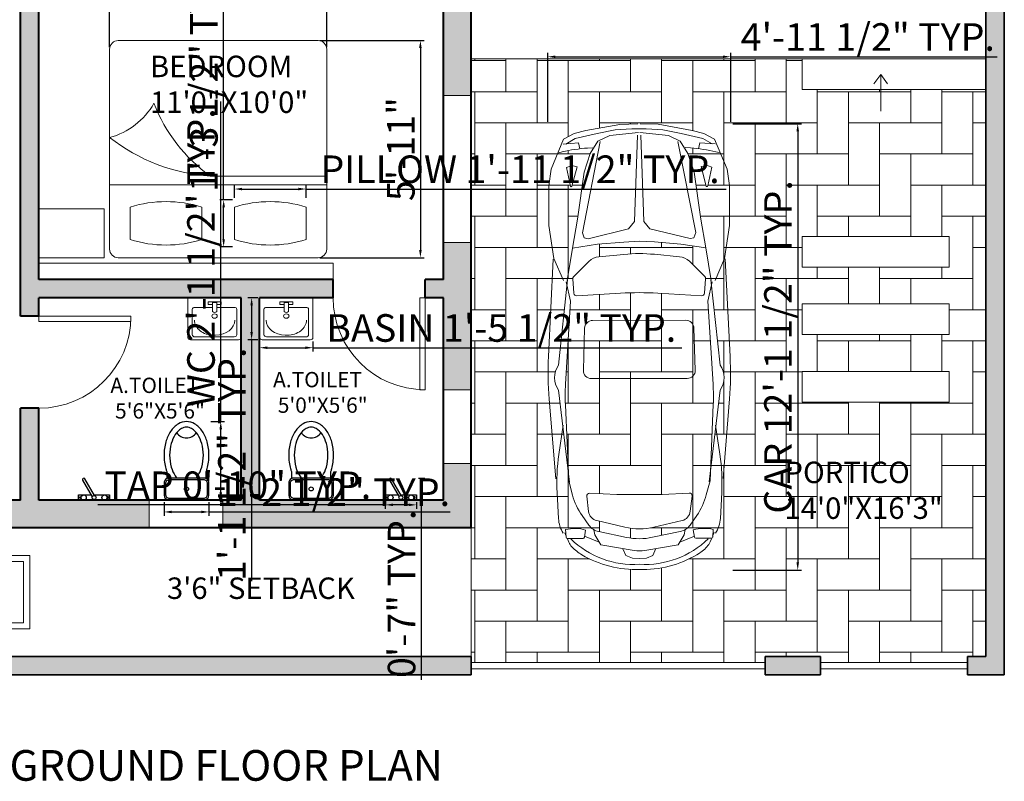
# Model space of a CAD drawing. Units: inches. Extents: x 2337 to 3570, y 1258 to 1938.
# Tile 2 of 30: x 2585 to 2906, y 1258 to 1507. Entities that reach past the tile are written whole.
import ezdxf

# ---------------------------------------------------------------- set-up
doc = ezdxf.new("R2010")
doc.units = ezdxf.units.IN
for name, color, linetype, lineweight in [('A-ANNO-DIMS', 2, 'Continuous', 18), ('A-ANNO-SYMB', 7, 'Continuous', 18), ('A-ANNO-TEXT', 7, 'Continuous', 18), ('A-ANNO-TITL', 7, 'Continuous', 30), ('A-AREA-IDEN', 7, 'Continuous', 18), ('A-DOOR', 4, 'Continuous', 20), ('A-FLOR-EDGE', 8, 'Continuous', 20), ('A-FLOR-PATT', 252, 'Continuous', 13), ('A-FLOR-STRS', 7, 'Continuous', 20), ('A-GLAZ', 4, 'Continuous', 18), ('A-WALL', 7, 'Continuous', 40), ('C-PROP', 7, 'Continuous', 35), ('furn', 8, 'Continuous', 18), ('L-PLNT-BEDS', 94, 'Continuous', 20), ('L-SITE-GATE', 4, 'Continuous', 18), ('L-SITE-VEHI', 8, 'Continuous', 18), ('Сантехника', 9, 'Continuous', 18)]:
    doc.layers.add(name, color=color, linetype=linetype, lineweight=lineweight)
doc.layers.add('A-WALL-PATT', color=18, linetype='Continuous', lineweight=13, true_color=0x000000)
doc.layers.add('C-PROP-PATT', color=251, linetype='Continuous', lineweight=13, true_color=0x636466)
doc.layers.add('SANTEH', color=7, linetype='Continuous')
doc.styles.get("Standard").update_dxf_attribs({"font": 'arial.ttf'})
doc.dimstyles.new('ISO-25', dxfattribs={"dimtxt": 9, "dimasz": 2.5, "dimexe": 1.25, "dimexo": 0.625, "dimtad": 1, "dimdec": 1, "dimlunit": 3, "dimtxsty": 'Standard', "dimcen": 2.5, "dimadec": 0, "dimazin": 0, "dimtfac": 1, "dimtdec": 1, "dimtmove": 0, "dimatfit": 3, "dimfxl": 1, "dimarcsym": 0})

# ---------------------------------------------------------------- blocks, each defined once
blk = doc.blocks.new('*U3')
for p, q in [((0, 0), (0, -6)), ((30, 0), (30, -6))]:
    blk.add_line(p, q)
blk.add_lwpolyline([(0, 0), (0, 30), (1.75, 30), (1.75, 0)], close=True)
blk.add_arc((0, 0), 30, 0, 90)
blk = doc.blocks.new('Rac7')
at = {"color": 0}
for p, q in [((-39473.6, -23808.4), (-38988.3, -23808.4)), ((-39500.6, -24232.1), (-39500.6, -23829.6)), ((-39456.5, -23859.1), (-39456.5, -24114.9)), ((-39032.4, -23838), (-39429.6, -23838)), ((-39221.1, -23854.9), (-39240.8, -23854.9)), ((-39005.4, -24114.9), (-39005.4, -23859.1)), ((-39005.4, -23859.1), (-39005.4, -23859.1)), ((-38961.3, -23829.6), (-38961.3, -24232.1)), ((-39252.5, -24185.9), (-39252.5, -24093.6)), ((-39209.4, -24185.9), (-39209.4, -24093.6)), ((-39429.6, -24136.1), (-39252.5, -24136.1)), ((-39297, -24164), (-39252.5, -24164)), ((-39297, -24193.5), (-39297, -24164)), ((-39164.9, -24193.5), (-39297, -24193.5)), ((-39252.5, -24185.9), (-39209.4, -24185.9)), ((-39209.4, -24136.1), (-39032.4, -24136.1)), ((-39209.4, -24164), (-39164.9, -24164)), ((-39164.9, -24164), (-39164.9, -24193.5)), ((-38961.3, -24232.1), (-39500.6, -24232.1))]:
    blk.add_line(p, q, dxfattribs=at)
at = {"color": 0, "extrusion": (0, 0, -1)}
for centre, major_axis, start_param, end_param in [((-39473.6, -23829.6), (-27, 0), 0, 1.570796), ((-38988.3, -23829.6), (-27, 0), 1.570796, 3.141593), ((-39429.6, -23859.1), (-27, 0), 0, 1.570796), ((-39240.8, -24007.4), (-194.1, 0), 0, 1.570796), ((-39221.1, -24007.4), (-194.1, 0), 1.570796, 3.141593), ((-39032.4, -23859.1), (-27, 0), 1.570796, 3.141593), ((-39231, -24104), (-25.3, 0), 0.552816, 2.588777), ((-39429.6, -24114.9), (-27, 0), -1.570796, 0), ((-39032.4, -24114.9), (-27, 0), -3.141593, -1.570796)]:
    blk.add_ellipse(centre, major_axis=major_axis, ratio=0.785714, start_param=start_param, end_param=end_param, dxfattribs=at)
blk.add_ellipse((-39231, -24048), major_axis=(-27.9, 0), ratio=0.785714, dxfattribs=at)
blk = doc.blocks.new('K10-44')
at = {"layer": 'SANTEH'}
for points in [[(-182, 222.6, 0.020439), (-174, 197.6), (-174, 134.8, 0.262987), (-198.2, 92), (-198.2, -8, 0.414214), (-148.2, -58), (151.8, -58, 0.414214), (201.8, -8), (201.8, 92, 0.262987), (177.6, 134.8), (177.6, 197.6, 0.020439), (185.6, 222.6, 0.067459), (201.8, 342, 0.067459), (185.6, 461.3, 0.079812), (143.2, 554.1, 0.107118), (73.7, 621.5, 0.139889), (1.8, 642, 0.139889), (-70.1, 621.5, 0.107118), (-139.6, 554.1, 0.079812), (-182, 461.3, 0.067459), (-198.2, 342, 0.067459)], [(-148.2, 127), (151.8, 127, -0.414214), (186.8, 92), (186.8, -8, -0.414214), (151.8, -43), (-148.2, -43, -0.414214), (-183.2, -8), (-183.2, 92, -0.414214)]]:
    blk.add_lwpolyline(points, format="xyb", close=True, dxfattribs=at)
for points in [[(89.9, 142, 0.027307), (101.6, 157.6, 0.079812), (137.4, 235.9, 0.067459), (151.8, 342, 0.067459), (137.4, 448, 0.079812), (101.6, 526.4, 0.107118), (47.3, 579, 0.139889), (1.8, 592, 0.139889), (-43.7, 579, 0.107118), (-98, 526.4, 0.079812), (-133.8, 448, 0.067459), (-148.2, 342, 0.067459), (-133.8, 235.9, 0.079812), (-98, 157.6, 0.027307), (-86.4, 142, 0.139889)], [(-174, 134.8, -0.136371), (-148.2, 142), (151.8, 142, -0.136371), (177.6, 134.8)]]:
    blk.add_lwpolyline(points, format="xyb", dxfattribs=at)
blk.add_circle((1.8, 42), 18.3, dxfattribs=at)
blk.add_arc((1.8, 601.6), 105.3, 213.89944, 326.10056, dxfattribs=at)
blk = doc.blocks.new('Faucet - kit sink top')
at = {"layer": 'SANTEH'}
for p, q in [((-5.5, -0.75), (-5.5, -1.25)), ((-4.94278, -0.75), (-5.5, -0.75)), ((-5.5, -1.25), (-4.94278, -1.25)), ((-0.14775, -1.7441), (3.56698, -8.1782)), ((4.43301, -7.6782), (0.71828, -1.2441)), ((4.94278, -0.75), (5.5, -0.75)), ((5.5, -1.25), (4.94278, -1.25)), ((5.5, -0.75), (5.5, -1.25))]:
    blk.add_line(p, q, dxfattribs=at)
blk.add_lwpolyline([(-0.00587, -2), (-6, -2), (-6, 0), (6, 0), (6, -2), (1.15195, -2)], dxfattribs=at)
for centre, radius in [((-4, -1), 1), ((4, -1), 1), ((0, -1), 0.75)]:
    blk.add_circle(centre, radius, dxfattribs=at)
blk.add_arc((4, -7.9282), 0.5, 210, 30, dxfattribs=at)
blk = doc.blocks.new('A$C4A3239E3')
for p, q in [((1.2507, 1.6335), (2.1522, 1.6799)), ((2.5445, 1.6742), (3.2816, 1.6148)), ((0.2661, 1.5794), (0.2592, 1.5495)), ((1.4425, 1.5023), (2.2313, 1.5881)), ((2.4629, 1.587), (3.3117, 1.4863)), ((2.7875, 1.5463), (3.0567, 1.5859)), ((3.4104, 1.6024), (3.6491, 1.5899)), ((0.1359, 1.4288), (0.1867, 1.515)), ((0.1752, 1.399), (0.1867, 1.5408)), ((0.3898, 1.477), (0.4021, 1.5106)), ((0.5758, 1.4596), (0.3963, 1.4117)), ((0.4021, 1.5106), (0.5754, 1.4741)), ((1.4497, 1.5063), (1.149, 1.4553)), ((1.4612, 1.5146), (1.6407, 1.4739)), ((1.6407, 1.4739), (2.4076, 1.5225)), ((2.597, 1.5244), (3.3012, 1.4943)), ((3.3012, 1.4943), (3.4322, 1.4598)), ((3.8218, 1.5205), (3.7519, 1.525)), ((3.7813, 1.5317), (3.8128, 1.5185)), ((3.8334, 1.3629), (3.8334, 1.5081)), ((3.8376, 1.5081), (3.8668, 1.4958)), ((0.0905, 1.2265), (0.1359, 1.4288)), ((0.2308, 1.3867), (0.1752, 1.399)), ((0.3963, 1.4117), (0.388, 1.4492)), ((1.2717, 1.3033), (1.4134, 1.4465)), ((1.4329, 1.4538), (1.567, 1.4437)), ((1.59, 1.4175), (1.5668, 1.0125)), ((3.6217, 1.372), (3.7108, 1.3099)), ((0.224, 1.314), (0.2207, 1.2655)), ((1.8899, 1.3452), (2.2788, 1.3576)), ((2.3557, 1.283), (2.3566, 0.3973)), ((3.4158, 1.3024), (3.4294, 1.0516)), ((3.4434, 1.3284), (3.584, 1.3121)), ((3.7558, 1.3393), (3.8231, 1.3506)), ((3.8137, 1.3503), (3.8686, 1.2144)), ((0.0565, 1.0588), (0.0905, 1.2265)), ((1.2074, 0.9801), (1.2293, 1.2125)), ((1.8186, 0.4085), (1.8178, 1.2708)), ((3.6693, 1.236), (3.7299, 0.9762)), ((3.7535, 1.2644), (3.8014, 1.2553)), ((3.7713, 1.2181), (3.8245, 0.9626)), ((3.8014, 1.2553), (3.8941, 1.199)), ((3.8941, 1.199), (3.9452, 0.89)), ((0.0481, 0.9038), (0.0565, 1.0588)), ((3.4294, 1.0516), (3.4292, 0.8428)), ((3.9292, 0.9941), (3.9933, 0.9668)), ((3.9933, 0.9668), (4.0172, 0.906)), ((3.4299, 0.6309), (3.4292, 0.8396)), ((4.0172, 0.906), (4.0211, 0.842)), ((4.0174, 0.7775), (4.0211, 0.8416)), ((0.0482, 0.7723), (0.0569, 0.6172)), ((3.8948, 0.4844), (3.9453, 0.7934)), ((3.9936, 0.7167), (4.0174, 0.7775)), ((1.2077, 0.6979), (1.23, 0.4656)), ((1.5911, 0.2613), (1.5671, 0.6662)), ((3.6701, 0.4469), (3.7301, 0.7068)), ((3.772, 0.465), (3.8248, 0.7206)), ((3.9295, 0.6893), (3.9936, 0.7167)), ((0.0569, 0.6172), (0.0912, 0.4496)), ((3.4167, 0.38), (3.4299, 0.6309)), ((3.8022, 0.4279), (3.8948, 0.4844)), ((3.8147, 0.3328), (3.8693, 0.4688)), ((0.0912, 0.4496), (0.1371, 0.2474)), ((0.2249, 0.3624), (0.2215, 0.4109)), ((1.2726, 0.3749), (1.4146, 0.232)), ((3.4444, 0.354), (3.585, 0.3707)), ((3.6228, 0.3107), (3.7117, 0.3731)), ((3.7543, 0.4187), (3.8022, 0.4279)), ((0.2318, 0.2897), (0.1763, 0.2773)), ((0.1763, 0.2773), (0.1881, 0.1355)), ((1.8909, 0.3342), (2.2798, 0.3226)), ((3.7568, 0.3438), (3.8241, 0.3326)), ((3.8345, 0.3203), (3.8347, 0.1751)), ((0.1371, 0.2474), (0.188, 0.1613)), ((0.3975, 0.2651), (0.3892, 0.2275)), ((0.3911, 0.1998), (0.4034, 0.1661)), ((0.5771, 0.2174), (0.3975, 0.2651)), ((0.4034, 0.1661), (0.5767, 0.203)), ((1.451, 0.1722), (1.1502, 0.2226)), ((1.4341, 0.2247), (1.5682, 0.235)), ((1.4625, 0.1639), (1.6419, 0.205)), ((1.6419, 0.205), (2.4089, 0.1579)), ((2.4644, 0.0936), (3.313, 0.1959)), ((2.5984, 0.1564), (3.3024, 0.1879)), ((3.3024, 0.1879), (3.4334, 0.2226)), ((3.8389, 0.1752), (3.8681, 0.1875)), ((0.2676, 0.0971), (0.2606, 0.127)), ((1.4438, 0.1762), (2.2328, 0.0919)), ((2.7889, 0.1349), (3.0581, 0.0958)), ((3.4119, 0.0799), (3.6506, 0.0929)), ((3.8231, 0.1627), (3.7532, 0.1581)), ((3.7826, 0.1514), (3.8141, 0.1647)), ((1.2522, 0.0446), (2.1538, 0)), ((2.5461, 0.0065), (3.2831, 0.0673))]:
    blk.add_line(p, q)
for points in [[(0, 0.8478), (0.0053, 1.0159), (0.0622, 1.3298), (0.0905, 1.4375), (0.1412, 1.5365), (0.4188, 1.6529), (0.572, 1.6743), (0.9399, 1.6743), (1.2458, 1.627), (1.4497, 1.5408)], [(0.0815, 0.8439), (0.1088, 1.11), (0.1609, 1.2182), (0.2737, 1.2906), (0.4463, 1.3472), (0.8811, 1.4091), (1.149, 1.4553), (1.1121, 1.224), (1.0933, 0.9813), (1.085, 0.8389)], [(0.1644, 1.198), (1.0072, 1.3636), (1.0537, 1.3462), (1.0619, 1.3117), (0.9706, 0.937), (0.9035, 0.8818), (0.106, 0.853)], [(0, 0.8281), (0.0056, 0.6601), (0.0632, 0.3462), (0.0916, 0.2386), (0.1426, 0.1398), (0.4204, 0.0239), (0.5737, 0.0028), (0.9415, 0.0032), (1.2473, 0.0511), (1.4511, 0.1377)], [(0.0815, 0.8322), (0.1094, 0.5662), (0.1616, 0.4581), (0.2746, 0.3859), (0.4473, 0.3296), (0.8822, 0.2683), (1.1502, 0.2226), (1.1128, 0.4539), (1.0936, 0.6965), (1.085, 0.8389)], [(0.1651, 0.4782), (1.0082, 0.314), (1.0547, 0.3316), (1.0628, 0.366), (0.9708, 0.7406), (0.9036, 0.7957), (0.1061, 0.8232)]]:
    blk.add_lwpolyline(points)
for centre, radius, start, end in [((2.3053, -1.296), 2.9798, 85.39524, 92.94517), ((1.7104, 1.2122), 1.4899, 166.91658, 176.08111), ((2.3463, 1.4226), 0.2016, 54.64918, 124.77695), ((3.3168, -0.183), 1.7879, 86.99981, 98.3676), ((3.6355, 1.3122), 0.278, 57.32995, 87.18237), ((0.4365, 1.46), 0.0497, 159.97873, 192.53841), ((0.5739, 1.4668), 0.00745, 284.96001, 78.11246), ((2.5206, -0.2618), 1.7879, 87.54913, 93.62371), ((3.2805, 0.8834), 0.596, 55.07004, 75.25506), ((4.0973, 1.4394), 0.3558, 166.09608, 196.35351), ((3.821, 1.5081), 0.0124, 0, 86.33043), ((3.2466, 0.8963), 0.8285, 356.24509, 44.51945), ((3.8091, 1.3584), 0.149, 46.38363, 67.20138), ((3.6181, 1.158), 0.4258, 30.45768, 46.38363), ((1.431, 1.429), 0.0248, 85.71507, 135.30465), ((1.5652, 1.4189), 0.0248, 356.72561, 85.71507), ((3.1325, 0.8724), 0.9892, 358.06945, 30.45768), ((1.3776, 1.1985), 0.149, 135.30465, 174.62136), ((1.8923, 1.2708), 0.0745, 91.82012, 179.9989), ((2.2812, 1.2831), 0.0745, 359.92446, 91.82012), ((3.4406, 1.3037), 0.0248, 83.37601, 183.11504), ((3.5726, 1.2134), 0.0993, 13.12265, 83.37601), ((3.6254, 1.1877), 0.149, 11.76937, 55.07004), ((3.821, 1.3629), 0.0124, 279.60772, 0), ((4.5417, 0.8423), 2.9798, 176.72561, 183.38736), ((2.6908, 0.8405), 1.4899, 174.62136, 185.49162), ((3.1495, 0.8409), 0.596, 346.99033, 13.12265), ((3.2411, 0.841), 0.596, 348.3436, 11.76937), ((1.2382, 0.8392), 1.1919, 176.89416, 183.21881), ((3.2467, 0.7858), 0.8285, 315.59352, 3.86789), ((3.6512, 0.8414), 0.298, 350.72464, 9.38834), ((3.1326, 0.8094), 0.9892, 329.65529, 2.04353), ((1.3783, 0.4799), 0.149, 185.49162, 224.80833), ((3.6261, 0.4951), 0.149, 305.04293, 348.3436), ((1.8931, 0.4086), 0.0745, 180.11408, 268.29286), ((2.2821, 0.397), 0.0745, 268.29286, 0.18852), ((3.4415, 0.3787), 0.0248, 176.99794, 276.73697), ((3.5733, 0.4693), 0.0993, 276.73697, 346.99033), ((1.7111, 0.4671), 1.4899, 184.03187, 193.1964), ((3.2806, 0.7987), 0.596, 284.85791, 305.04293), ((4.0985, 0.2443), 0.3558, 163.75946, 194.01689), ((3.822, 0.3203), 0.0124, 0.11298, 80.50526), ((3.6188, 0.5248), 0.4258, 313.72935, 329.65529), ((0.4377, 0.2169), 0.0497, 167.57457, 200.13424), ((0.5752, 0.2102), 0.00745, 282.00051, 75.15297), ((1.4322, 0.2495), 0.0248, 224.80833, 274.3979), ((1.5663, 0.2598), 0.0248, 274.3979, 3.38736), ((3.8101, 0.3247), 0.149, 292.9116, 313.72935), ((2.3474, 0.2577), 0.2016, 235.33603, 305.46379), ((2.5184, 1.9425), 1.7879, 266.48926, 272.56385), ((3.3148, 1.8652), 1.7879, 261.74537, 273.11317), ((3.6364, 0.3706), 0.278, 272.9306, 302.78303), ((3.8223, 0.1751), 0.0124, 273.78255, 0.11298), ((2.3011, 2.9762), 2.9798, 267.1678, 274.71773)]:
    blk.add_arc(centre, radius, start, end)
blk = doc.blocks.new('STAIR-UP-ARROW')
for p, q in [((2.25, 12), (2.25, 0)), ((2.25, 0), (0, 3.01)), ((2.25, 0), (4.5, 3.01))]:
    blk.add_line(p, q)
blk = doc.blocks.new('BED-PILLOW')
for p, q in [((0, 1.77), (0, 12.4)), ((23.39, 12.4), (23.39, 1.77))]:
    blk.add_line(p, q)
for centre, start, end in [((11.69, -25.3), 72.7687, 107.2313), ((11.69, 39.47), 252.7687, 287.2313)]:
    blk.add_arc(centre, 39.47, start, end)
blk = doc.blocks.new('PLANTER-132X24IN')
for points in [[(0, 24), (132, 24), (132, 0), (0, 0)], [(2, 22), (130, 22), (130, 2), (2, 2)]]:
    blk.add_lwpolyline(points, close=True)
blk = doc.blocks.new('*D58')
at = {"layer": 'A-ANNO-DIMS', "color": 0, "lineweight": -2, "transparency": 16777216}
for p, q in [((2662.84, 1401.83), (2662.84, 1398.59)), ((2680.23, 1401.83), (2680.23, 1398.59)), ((2665.34, 1399.84), (2677.73, 1399.84)), ((2680.23, 1399.84), (2800.63, 1399.84))]:
    blk.add_line(p, q, dxfattribs=at)
at = {"layer": 'A-ANNO-DIMS', "color": 0, "transparency": 16777216}
for points in [[(2665.34, 1400.26), (2665.34, 1399.43), (2662.84, 1399.84)], [(2677.73, 1400.26), (2677.73, 1399.43), (2680.23, 1399.84)]]:
    blk.add_solid(points, dxfattribs=at)
at = {"layer": 'Defpoints', "color": 0, "transparency": 16777216}
for p in [(2662.84, 1402.45), (2680.23, 1402.45), (2680.23, 1399.84)]:
    blk.add_point(p, dxfattribs=at)
at = {"layer": 'A-ANNO-DIMS', "color": 0, "transparency": 16777216, "insert": (2741.68, 1405.12), "char_height": 9, "attachment_point": 5}
blk.add_mtext('BASIN 1\'-5 1/2" TYP.', dxfattribs=at)
blk = doc.blocks.new('*D59')
at = {"layer": 'A-ANNO-DIMS', "color": 0, "lineweight": -2, "transparency": 16777216}
for p, q in [((2662.21, 1416.12), (2658.98, 1416.12)), ((2660.23, 1413.62), (2660.23, 1404.95)), ((2662.21, 1402.45), (2658.98, 1402.45)), ((2660.23, 1402.45), (2660.23, 1323.72))]:
    blk.add_line(p, q, dxfattribs=at)
at = {"layer": 'A-ANNO-DIMS', "color": 0, "transparency": 16777216}
for points in [[(2659.81, 1413.62), (2660.64, 1413.62), (2660.23, 1416.12)], [(2659.81, 1404.95), (2660.64, 1404.95), (2660.23, 1402.45)]]:
    blk.add_solid(points, dxfattribs=at)
at = {"layer": 'Defpoints', "color": 0, "transparency": 16777216}
for p in [(2662.84, 1416.12), (2660.23, 1402.45), (2662.84, 1402.45)]:
    blk.add_point(p, dxfattribs=at)
at = {"layer": 'A-ANNO-DIMS', "color": 0, "transparency": 16777216, "insert": (2654.95, 1361.83), "char_height": 9, "attachment_point": 5, "rotation": 90}
blk.add_mtext('1\'-1 1/2" TYP.', dxfattribs=at)
blk = doc.blocks.new('*D60')
at = {"layer": 'A-ANNO-DIMS', "color": 0, "lineweight": -2, "transparency": 16777216}
for p, q in [((2650.15, 1375.76), (2650.15, 1480.15)), ((2646.93, 1375.76), (2651.4, 1375.76)), ((2650.15, 1352.62), (2650.15, 1373.26)), ((2646.93, 1350.12), (2651.4, 1350.12))]:
    blk.add_line(p, q, dxfattribs=at)
at = {"layer": 'A-ANNO-DIMS', "color": 0, "transparency": 16777216}
for points in [[(2649.73, 1373.26), (2650.57, 1373.26), (2650.15, 1375.76)], [(2649.73, 1352.62), (2650.57, 1352.62), (2650.15, 1350.12)]]:
    blk.add_solid(points, dxfattribs=at)
at = {"layer": 'Defpoints', "color": 0, "transparency": 16777216}
for p in [(2646.3, 1375.76), (2650.15, 1375.76), (2646.3, 1350.12)]:
    blk.add_point(p, dxfattribs=at)
at = {"layer": 'A-ANNO-DIMS', "color": 0, "transparency": 16777216, "insert": (2644.87, 1429.21), "char_height": 9, "attachment_point": 5, "rotation": 90}
blk.add_mtext('WC 2\'-1 1/2" TYP.', dxfattribs=at)
blk = doc.blocks.new('*D61')
at = {"layer": 'A-ANNO-DIMS', "color": 0, "lineweight": -2, "transparency": 16777216}
for p, q in [((2631.65, 1349.49), (2631.65, 1345.02)), ((2646.3, 1349.49), (2646.3, 1345.02)), ((2634.15, 1346.27), (2643.8, 1346.27)), ((2646.3, 1346.27), (2725.04, 1346.27))]:
    blk.add_line(p, q, dxfattribs=at)
at = {"layer": 'A-ANNO-DIMS', "color": 0, "transparency": 16777216}
for points in [[(2634.15, 1346.69), (2634.15, 1345.85), (2631.65, 1346.27)], [(2643.8, 1346.69), (2643.8, 1345.85), (2646.3, 1346.27)]]:
    blk.add_solid(points, dxfattribs=at)
at = {"layer": 'Defpoints', "color": 0, "transparency": 16777216}
for p in [(2631.65, 1350.12), (2646.3, 1350.12), (2646.3, 1346.27)]:
    blk.add_point(p, dxfattribs=at)
at = {"layer": 'A-ANNO-DIMS', "color": 0, "transparency": 16777216, "insert": (2686.92, 1351.55), "char_height": 9, "attachment_point": 5}
blk.add_mtext('1\'-2 1/2" TYP.', dxfattribs=at)
blk = doc.blocks.new('*D62')
at = {"layer": 'A-ANNO-DIMS', "color": 0, "lineweight": -2, "transparency": 16777216}
for p, q in [((2703.85, 1349.49), (2703.85, 1347.34)), ((2714.01, 1349.49), (2714.01, 1347.34)), ((2703.85, 1348.59), (2610.07, 1348.59)), ((2711.51, 1348.59), (2706.35, 1348.59))]:
    blk.add_line(p, q, dxfattribs=at)
at = {"layer": 'A-ANNO-DIMS', "color": 0, "transparency": 16777216}
for points in [[(2706.35, 1349.01), (2706.35, 1348.17), (2703.85, 1348.59)], [(2711.51, 1349.01), (2711.51, 1348.17), (2714.01, 1348.59)]]:
    blk.add_solid(points, dxfattribs=at)
at = {"layer": 'Defpoints', "color": 0, "transparency": 16777216}
for p in [(2703.85, 1350.12), (2714.01, 1350.12), (2703.85, 1348.59)]:
    blk.add_point(p, dxfattribs=at)
at = {"layer": 'A-ANNO-DIMS', "color": 0, "transparency": 16777216, "insert": (2655.71, 1353.81), "char_height": 9, "attachment_point": 5}
blk.add_mtext('TAP 0\'-10" TYP.', dxfattribs=at)
blk = doc.blocks.new('*D63')
at = {"layer": 'A-ANNO-DIMS', "color": 0, "lineweight": -2, "transparency": 16777216}
for p, q in [((2714.64, 1357.31), (2716.79, 1357.31)), ((2715.54, 1354.81), (2715.54, 1352.62)), ((2714.64, 1350.12), (2716.79, 1350.12)), ((2715.54, 1350.12), (2715.54, 1291.51))]:
    blk.add_line(p, q, dxfattribs=at)
at = {"layer": 'A-ANNO-DIMS', "color": 0, "transparency": 16777216}
for points in [[(2715.12, 1354.81), (2715.95, 1354.81), (2715.54, 1357.31)], [(2715.12, 1352.62), (2715.95, 1352.62), (2715.54, 1350.12)]]:
    blk.add_solid(points, dxfattribs=at)
at = {"layer": 'Defpoints', "color": 0, "transparency": 16777216}
for p in [(2714.01, 1357.31), (2714.01, 1350.12), (2715.54, 1350.12)]:
    blk.add_point(p, dxfattribs=at)
at = {"layer": 'A-ANNO-DIMS', "color": 0, "transparency": 16777216, "insert": (2710.32, 1319.56), "char_height": 9, "attachment_point": 5, "rotation": 90}
blk.add_mtext('0\'-7" TYP.', dxfattribs=at)
blk = doc.blocks.new('*D64')
at = {"layer": 'A-ANNO-DIMS', "color": 0, "lineweight": -2, "transparency": 16777216}
for p, q in [((2817.21, 1472.91), (2839.68, 1472.91)), ((2838.43, 1470.41), (2838.43, 1329.8)), ((2817.21, 1327.3), (2839.68, 1327.3))]:
    blk.add_line(p, q, dxfattribs=at)
at = {"layer": 'A-ANNO-DIMS', "color": 0, "transparency": 16777216}
for points in [[(2838.01, 1470.41), (2838.84, 1470.41), (2838.43, 1472.91)], [(2838.01, 1329.8), (2838.84, 1329.8), (2838.43, 1327.3)]]:
    blk.add_solid(points, dxfattribs=at)
at = {"layer": 'Defpoints', "color": 0, "transparency": 16777216}
for p in [(2816.59, 1472.91), (2816.59, 1327.3), (2838.43, 1327.3)]:
    blk.add_point(p, dxfattribs=at)
at = {"layer": 'A-ANNO-DIMS', "color": 0, "transparency": 16777216, "insert": (2833.15, 1400.11), "char_height": 9, "attachment_point": 5, "rotation": 90}
blk.add_mtext('CAR 12\'-1 1/2" TYP.', dxfattribs=at)
blk = doc.blocks.new('*D65')
at = {"layer": 'A-ANNO-DIMS', "color": 0, "lineweight": -2, "transparency": 16777216}
for p, q in [((2756.86, 1473.54), (2756.86, 1496)), ((2759.36, 1494.75), (2814.09, 1494.75)), ((2816.59, 1473.54), (2816.59, 1496)), ((2816.59, 1494.75), (2903.52, 1494.75))]:
    blk.add_line(p, q, dxfattribs=at)
at = {"layer": 'A-ANNO-DIMS', "color": 0, "transparency": 16777216}
for points in [[(2759.36, 1495.17), (2759.36, 1494.34), (2756.86, 1494.75)], [(2814.09, 1495.17), (2814.09, 1494.34), (2816.59, 1494.75)]]:
    blk.add_solid(points, dxfattribs=at)
at = {"layer": 'Defpoints', "color": 0, "transparency": 16777216}
for p in [(2816.59, 1494.75), (2756.86, 1472.91), (2816.59, 1472.91)]:
    blk.add_point(p, dxfattribs=at)
at = {"layer": 'A-ANNO-DIMS', "color": 0, "transparency": 16777216, "insert": (2861.3, 1500.03), "char_height": 9, "attachment_point": 5}
blk.add_mtext('4\'-11 1/2" TYP.', dxfattribs=at)
blk = doc.blocks.new('*D66')
at = {"layer": 'A-ANNO-DIMS', "color": 0, "lineweight": -2, "transparency": 16777216}
for p, q in [((2654.61, 1448.73), (2654.61, 1452.86)), ((2678, 1448.73), (2678, 1452.86)), ((2657.11, 1451.61), (2675.5, 1451.61)), ((2678, 1451.61), (2815.12, 1451.61))]:
    blk.add_line(p, q, dxfattribs=at)
at = {"layer": 'A-ANNO-DIMS', "color": 0, "transparency": 16777216}
for points in [[(2657.11, 1452.03), (2657.11, 1451.19), (2654.61, 1451.61)], [(2675.5, 1452.03), (2675.5, 1451.19), (2678, 1451.61)]]:
    blk.add_solid(points, dxfattribs=at)
at = {"layer": 'Defpoints', "color": 0, "transparency": 16777216}
for p in [(2678, 1451.61), (2654.61, 1448.1), (2678, 1448.1)]:
    blk.add_point(p, dxfattribs=at)
at = {"layer": 'A-ANNO-DIMS', "color": 0, "transparency": 16777216, "insert": (2747.81, 1456.89), "char_height": 9, "attachment_point": 5}
blk.add_mtext('PILLOW 1\'-11 1/2" TYP.', dxfattribs=at)
blk = doc.blocks.new('*D67')
at = {"layer": 'A-ANNO-DIMS', "color": 0, "lineweight": -2, "transparency": 16777216}
for p, q in [((2651.1, 1448.1), (2651.1, 1526.84)), ((2653.98, 1448.1), (2649.85, 1448.1)), ((2651.1, 1435.25), (2651.1, 1445.6)), ((2653.98, 1432.75), (2649.85, 1432.75))]:
    blk.add_line(p, q, dxfattribs=at)
at = {"layer": 'A-ANNO-DIMS', "color": 0, "transparency": 16777216}
for points in [[(2650.68, 1445.6), (2651.52, 1445.6), (2651.1, 1448.1)], [(2650.68, 1435.25), (2651.52, 1435.25), (2651.1, 1432.75)]]:
    blk.add_solid(points, dxfattribs=at)
at = {"layer": 'Defpoints', "color": 0, "transparency": 16777216}
for p in [(2651.1, 1448.1), (2654.61, 1448.1), (2654.61, 1432.75)]:
    blk.add_point(p, dxfattribs=at)
at = {"layer": 'A-ANNO-DIMS', "color": 0, "transparency": 16777216, "insert": (2645.82, 1488.72), "char_height": 9, "attachment_point": 5, "rotation": 90}
blk.add_mtext('1\'-3 1/2" TYP.', dxfattribs=at)
blk = doc.blocks.new('*D118')
at = {"layer": 'A-ANNO-DIMS', "color": 0, "lineweight": -2, "transparency": 16777216}
for p, q in [((2613.87, 1497.86), (2613.87, 1927.77)), ((2684.73, 1497.86), (2684.73, 1927.77)), ((2616.37, 1926.52), (2682.23, 1926.52))]:
    blk.add_line(p, q, dxfattribs=at)
at = {"layer": 'A-ANNO-DIMS', "color": 0, "transparency": 16777216}
for points in [[(2616.37, 1926.93), (2616.37, 1926.1), (2613.87, 1926.52)], [(2682.23, 1926.93), (2682.23, 1926.1), (2684.73, 1926.52)]]:
    blk.add_solid(points, dxfattribs=at)
at = {"layer": 'Defpoints', "color": 0, "transparency": 16777216}
for p in [(2684.73, 1926.52), (2613.87, 1497.23), (2684.73, 1497.23)]:
    blk.add_point(p, dxfattribs=at)
at = {"layer": 'A-ANNO-DIMS', "color": 0, "transparency": 16777216, "insert": (2649.3, 1931.74), "char_height": 9, "attachment_point": 5}
blk.add_mtext('5\'-11"', dxfattribs=at)
blk = doc.blocks.new('*D119')
at = {"layer": 'A-ANNO-DIMS', "color": 0, "lineweight": -2, "transparency": 16777216}
for p, q in [((2682.52, 1500.07), (2716.55, 1500.07)), ((2715.3, 1497.57), (2715.3, 1431.7)), ((2682.52, 1429.2), (2716.55, 1429.2))]:
    blk.add_line(p, q, dxfattribs=at)
at = {"layer": 'A-ANNO-DIMS', "color": 0, "transparency": 16777216}
for points in [[(2714.88, 1497.57), (2715.72, 1497.57), (2715.3, 1500.07)], [(2714.88, 1431.7), (2715.72, 1431.7), (2715.3, 1429.2)]]:
    blk.add_solid(points, dxfattribs=at)
at = {"layer": 'Defpoints', "color": 0, "transparency": 16777216}
for p in [(2681.9, 1500.07), (2681.9, 1429.2), (2715.3, 1429.2)]:
    blk.add_point(p, dxfattribs=at)
at = {"layer": 'A-ANNO-DIMS', "color": 0, "transparency": 16777216, "insert": (2710.08, 1464.64), "char_height": 9, "attachment_point": 5, "rotation": 90}
blk.add_mtext('5\'-11"', dxfattribs=at)

msp = doc.modelspace()

# ---------------------------------------------------------------- hatches: boundary and pattern name
at = {"layer": 'A-FLOR-PATT', "transparency": 33554687}
h = msp.add_hatch(dxfattribs=at)
h.set_pattern_fill('AR-HBONE', color=256, scale=0.1, angle=45)
h.paths.add_polyline_path([(2899.84, 1484.12), (2839.84, 1484.12), (2839.84, 1494.12), (2731.84, 1494.12), (2731.84, 1341.12), (2731.84, 1299.12), (2731.84, 1297.12), (2827.84, 1297.12), (2827.84, 1299.12), (2845.84, 1299.12), (2845.84, 1297.12), (2893.84, 1297.12), (2893.84, 1299.12), (2899.84, 1299.12)])
h.paths.add_polyline_path([(2813.17, 1463.44), (2811.75, 1463.77, 0.040009), (2803.44, 1465.01), (2801.4, 1465.15), (2802.62, 1463.26), (2804.61, 1457.17), (2806.8, 1441.83), (2808.43, 1432.38), (2800.27, 1433.68), (2791.7, 1434.34), (2786.68, 1434.64), (2781.66, 1434.33), (2773.1, 1433.66), (2764.94, 1432.34), (2766.55, 1441.79), (2768.71, 1457.13), (2770.7, 1463.22), (2771.91, 1465.12), (2769.87, 1464.98, 0.040009), (2761.57, 1463.72), (2760.14, 1463.39), (2762.02, 1467.88), (2765.51, 1469.68), (2769.3, 1470.68), (2780.37, 1472.71), (2786.65, 1472.92), (2792.92, 1472.73), (2804, 1470.72), (2807.8, 1469.72), (2811.29, 1467.93)], flags=16)
h.paths.add_polyline_path([(2810.38, 1458.73), (2809.09, 1452.61, -0.789416), (2808.58, 1452.6), (2806.89, 1458.93), (2808.71, 1459.34)], flags=16)
h.paths.add_polyline_path([(2839.84, 1436.12), (2887.84, 1436.12), (2887.84, 1426.12), (2839.84, 1426.12)], flags=16)
h.paths.add_polyline_path([(2803.06, 1428.05), (2808.4, 1422.77), (2808.02, 1417.63, -0.409057), (2807.09, 1416.82), (2792.8, 1417.64, 0.029076), (2780.59, 1417.63), (2766.3, 1416.78, -0.409057), (2765.38, 1417.59), (2764.98, 1422.73), (2770.31, 1428.02, -0.173254), (2773.51, 1429.52), (2781.71, 1430.31, -0.047466), (2791.66, 1430.32), (2799.86, 1429.55, -0.173254)], flags=16)
h.paths.add_polyline_path([(2813.11, 1394.2, -0.315912), (2813.07, 1386.03), (2809.93, 1359.6), (2809.8, 1356.46), (2808.58, 1351.84, -0.088302), (2805.49, 1345.15), (2803.29, 1342.01, -0.105467), (2801.69, 1340.52), (2801.37, 1338.82), (2799.93, 1336.44), (2804.68, 1338.36), (2804.33, 1340.42, -0.132795), (2810.88, 1340.56), (2810.7, 1337.68), (2810.35, 1337.68), (2809.85, 1336.51, -0.091085), (2808.81, 1334.92, -0.069602), (2805.55, 1332.33, -0.141553), (2786.79, 1327.53, -0.141553), (2768.01, 1332.29, -0.069602), (2764.75, 1334.87, -0.091085), (2763.7, 1336.46), (2763.2, 1337.64, -0.354729), (2762.83, 1338.05), (2762.66, 1340.51, -0.132795), (2769.22, 1340.39), (2768.87, 1338.33), (2773.63, 1336.42), (2772.18, 1338.79), (2771.86, 1340.49, -0.105467), (2770.25, 1341.98), (2768.05, 1345.12, -0.088302), (2764.94, 1351.8), (2763.72, 1356.42), (2763.58, 1359.56), (2760.39, 1385.98, -0.315912), (2760.33, 1394.15), (2763.12, 1420.24), (2764.32, 1414.99), (2762.66, 1387.93, 0.026512), (2762.6, 1381.25), (2763.72, 1356.42), (2764.94, 1351.8, 0.088302), (2768.05, 1345.12), (2770.25, 1341.98, 0.191215), (2773.49, 1339.85), (2782.51, 1337.99, 0.102572), (2791.04, 1338), (2800.06, 1339.88, 0.191215), (2803.29, 1342.01), (2805.49, 1345.15, 0.088302), (2808.58, 1351.84), (2809.8, 1356.46), (2810.86, 1381.3, 0.026512), (2810.79, 1387.98), (2809.08, 1415.04), (2810.27, 1420.29)], flags=16)
h.paths.add_polyline_path([(2839.84, 1414.12), (2887.84, 1414.12), (2887.84, 1404.12), (2839.84, 1404.12)], flags=16)
h.paths.add_polyline_path([(2766.44, 1458.89), (2764.76, 1452.56, -0.789416), (2764.25, 1452.57), (2762.95, 1458.68), (2764.61, 1459.29)], flags=16)
h.paths.add_polyline_path([(2768.47, 1392.49), (2768.88, 1406.21, -0.405226), (2771.5, 1408.76), (2771.5, 1408.76, 0.40508), (2768.88, 1406.21), (2768.47, 1392.49, 0.423258), (2771.1, 1389.78), (2771.1, 1389.78, -0.423258)], flags=16)
h.paths.add_polyline_path([(2839.84, 1392.12), (2887.84, 1392.12), (2887.84, 1382.12), (2839.84, 1382.12)], flags=16)
h.paths.add_polyline_path([(2803.03, 1352.42, -0.464922), (2803.95, 1351.44), (2803.37, 1346.48, -0.316515), (2800.69, 1343.47), (2791.53, 1341.34, -0.11452), (2782.02, 1341.33), (2772.85, 1343.45, -0.316515), (2770.16, 1346.45), (2769.58, 1351.41, -0.464922), (2770.49, 1352.38), (2779.34, 1351.92), (2786.76, 1351.95), (2794.18, 1351.94)], flags=16)
h.paths.add_polyline_path([(2792.17, 1334.35), (2791.19, 1332.04), (2789.05, 1331.2), (2786.78, 1331.06), (2784.52, 1331.2), (2782.37, 1332.04), (2781.38, 1334.34), (2785.08, 1333.74, 0.081616), (2788.48, 1333.74)], flags=0)
h.paths.add_polyline_path([(2831.29, 1340.04), (2884.62, 1340.04), (2884.62, 1366.16), (2831.29, 1366.16)], flags=24)
at = {"layer": 'A-WALL-PATT'}
h = msp.add_hatch(color=256, dxfattribs=at)
h.dxf.hatch_style = 1
h.paths.add_polyline_path([(2671.84, 1857.12), (2455.84, 1857.12), (2455.84, 1824.12), (2464.84, 1824.12), (2464.84, 1848.12), (2671.84, 1848.12)])
h.paths.add_polyline_path([(2566.84, 1764.12), (2464.84, 1764.12), (2464.84, 1788.12), (2455.84, 1788.12), (2455.84, 1743.12), (2464.84, 1743.12), (2464.84, 1755.12), (2566.84, 1755.12)])
h.paths.add_polyline_path([(2683.84, 1761.12), (2683.84, 1764.12), (2602.84, 1764.12), (2602.84, 1755.12), (2608.84, 1755.12), (2608.84, 1701.12), (2662.84, 1701.12), (2662.84, 1605.12), (2671.84, 1605.12), (2671.84, 1713.12), (2662.84, 1713.12), (2662.84, 1707.12), (2614.84, 1707.12), (2614.84, 1755.12), (2662.84, 1755.12), (2662.84, 1749.12), (2671.84, 1749.12), (2671.84, 1755.12), (2683.84, 1755.12)])
h.paths.add_polyline_path([(2464.84, 1707.12), (2455.84, 1707.12), (2455.84, 1617.12), (2464.84, 1617.12), (2464.84, 1635.12), (2506.84, 1635.12), (2506.84, 1641.12), (2464.84, 1641.12)])
h.paths.add_polyline_path([(2542.84, 1551.12), (2464.84, 1551.12), (2464.84, 1569.12), (2455.84, 1569.12), (2455.84, 1518.12), (2464.84, 1518.12), (2464.84, 1542.12), (2542.84, 1542.12)])
h.paths.add_polyline_path([(2464.84, 1482.12), (2455.84, 1482.12), (2455.84, 1410.12), (2464.84, 1410.12)])
h.paths.add_polyline_path([(2626.84, 1350.12), (2590.84, 1350.12), (2590.84, 1380.12), (2584.84, 1380.12), (2584.84, 1350.12), (2464.84, 1350.12), (2464.84, 1374.12), (2455.84, 1374.12), (2455.84, 1341.12), (2626.84, 1341.12)])
h.paths.add_polyline_path([(2662.84, 1416.12), (2686.84, 1416.12), (2686.84, 1422.12), (2590.84, 1422.12), (2590.84, 1542.12), (2680.84, 1542.12), (2680.84, 1551.12), (2671.84, 1551.12), (2671.84, 1557.12), (2662.84, 1557.12), (2662.84, 1551.12), (2578.84, 1551.12), (2578.84, 1542.12), (2584.84, 1542.12), (2584.84, 1410.12), (2590.84, 1410.12), (2590.84, 1416.12), (2656.84, 1416.12), (2656.84, 1350.12), (2650.84, 1350.12), (2650.84, 1341.12), (2731.84, 1341.12), (2731.84, 1362.12), (2722.84, 1362.12), (2722.84, 1350.12), (2662.84, 1350.12)])
h.paths.add_polyline_path([(2731.84, 1434.12), (2722.84, 1434.12), (2722.84, 1422.12), (2716.84, 1422.12), (2716.84, 1416.12), (2722.84, 1416.12), (2722.84, 1386.12), (2731.84, 1386.12)], flags=17)
h.paths.add_polyline_path([(2731.84, 1542.12), (2752.84, 1542.12), (2752.84, 1551.12), (2716.84, 1551.12), (2716.84, 1545.12), (2716.84, 1542.12), (2722.84, 1542.12), (2722.84, 1482.12), (2731.84, 1482.12)])
h.paths.add_polyline_path([(2809.84, 1551.12), (2788.84, 1551.12), (2788.84, 1542.12), (2809.84, 1542.12), (2809.84, 1548.12)])
h.paths.add_polyline_path([(2872.84, 1647.12), (2863.84, 1647.12), (2863.84, 1551.12), (2857.84, 1551.12), (2857.84, 1548.12), (2857.84, 1542.12), (2872.84, 1542.12)])
h.paths.add_polyline_path([(2872.84, 1764.12), (2827.84, 1764.12), (2827.84, 1755.12), (2863.84, 1755.12), (2863.84, 1719.12), (2872.84, 1719.12)])
h.paths.add_polyline_path([(2755.84, 1764.12), (2719.84, 1764.12), (2719.84, 1755.12), (2755.84, 1755.12)])
at = {"layer": 'C-PROP-PATT'}
h = msp.add_hatch(color=256, dxfattribs=at)
h.dxf.hatch_style = 1
h.paths.add_polyline_path([(2905.84, 1893.12), (2425.84, 1893.12), (2425.84, 1293.12), (2731.84, 1293.12), (2731.84, 1299.12), (2431.84, 1299.12), (2431.84, 1887.12), (2899.84, 1887.12), (2899.84, 1875.12), (2905.84, 1875.12)])
h.paths.add_polyline_path([(2845.84, 1299.12), (2827.84, 1299.12), (2827.84, 1293.12), (2845.84, 1293.12)], flags=17)
h.paths.add_polyline_path([(2905.84, 1779.12), (2899.84, 1779.12), (2899.84, 1299.12), (2893.84, 1299.12), (2893.84, 1293.12), (2905.84, 1293.12)], flags=17)

# ---------------------------------------------------------------- linework, layer by layer
at = {"layer": 'A-FLOR-EDGE'}
for p, q in [((2899.84, 1494.12), (2731.84, 1494.12)), ((2731.84, 1341.12), (2731.84, 1299.12))]:
    msp.add_line(p, q, dxfattribs=at)
for points in [[(2839.84, 1436.12), (2887.84, 1436.12), (2887.84, 1426.12), (2839.84, 1426.12)], [(2839.84, 1414.12), (2887.84, 1414.12), (2887.84, 1404.12), (2839.84, 1404.12)], [(2839.84, 1392.12), (2887.84, 1392.12), (2887.84, 1382.12), (2839.84, 1382.12)]]:
    msp.add_lwpolyline(points, close=True, dxfattribs=at)
at = {"layer": 'A-FLOR-STRS'}
for p, q in [((2839.84, 1484.12), (2839.84, 1494.12)), ((2899.84, 1484.12), (2839.84, 1484.12))]:
    msp.add_line(p, q, dxfattribs=at)
at = {"layer": 'A-GLAZ'}
for p, q in [((2731.84, 1482.12), (2722.84, 1482.12)), ((2731.84, 1434.12), (2722.84, 1434.12)), ((2731.84, 1386.12), (2722.84, 1386.12)), ((2731.84, 1362.12), (2722.84, 1362.12)), ((2626.84, 1341.12), (2626.84, 1350.12)), ((2650.84, 1341.12), (2650.84, 1350.12))]:
    msp.add_line(p, q, dxfattribs=at)
at = {"layer": 'A-WALL'}
for p, q in [((2584.84, 1410.12), (2584.84, 1542.12)), ((2590.84, 1422.12), (2590.84, 1542.12)), ((2722.84, 1422.12), (2722.84, 1542.12)), ((2731.84, 1341.12), (2731.84, 1542.12)), ((2686.84, 1422.12), (2590.84, 1422.12)), ((2686.84, 1416.12), (2686.84, 1422.12)), ((2722.84, 1422.12), (2716.84, 1422.12)), ((2716.84, 1416.12), (2716.84, 1422.12)), ((2656.84, 1416.12), (2590.84, 1416.12)), ((2590.84, 1410.12), (2590.84, 1416.12)), ((2656.84, 1350.12), (2656.84, 1416.12)), ((2686.84, 1416.12), (2662.84, 1416.12)), ((2662.84, 1350.12), (2662.84, 1416.12)), ((2722.84, 1416.12), (2716.84, 1416.12)), ((2722.84, 1350.12), (2722.84, 1416.12)), ((2590.84, 1410.12), (2584.84, 1410.12)), ((2590.84, 1380.12), (2584.84, 1380.12)), ((2584.84, 1350.12), (2584.84, 1380.12)), ((2590.84, 1350.12), (2590.84, 1380.12)), ((2584.84, 1350.12), (2464.84, 1350.12)), ((2656.84, 1350.12), (2590.84, 1350.12)), ((2722.84, 1350.12), (2662.84, 1350.12)), ((2731.84, 1341.12), (2455.84, 1341.12))]:
    msp.add_line(p, q, dxfattribs=at)
at = {"layer": 'C-PROP'}
for p, q in [((2899.84, 1779.12), (2899.84, 1299.12)), ((2905.84, 1779.12), (2905.84, 1293.12)), ((2731.84, 1299.12), (2431.84, 1299.12)), ((2731.84, 1299.12), (2731.84, 1293.12)), ((2827.84, 1299.12), (2827.84, 1293.12)), ((2845.84, 1299.12), (2845.84, 1293.12)), ((2899.84, 1299.12), (2893.84, 1299.12)), ((2893.84, 1299.12), (2893.84, 1293.12)), ((2731.84, 1293.12), (2425.84, 1293.12)), ((2845.84, 1293.12), (2827.84, 1293.12)), ((2905.84, 1293.12), (2893.84, 1293.12))]:
    msp.add_line(p, q, dxfattribs=at)
msp.add_lwpolyline([(2845.84, 1299.12), (2827.84, 1299.12)], dxfattribs=at)
at = {"layer": 'furn'}
for p, q in [((2613.87, 1497.23), (2613.87, 1432.04)), ((2681.9, 1500.07), (2616.7, 1500.07)), ((2684.73, 1432.04), (2684.73, 1497.23)), ((2684.73, 1455.76), (2646.77, 1455.76)), ((2684.73, 1452.93), (2613.87, 1452.93)), ((2590.84, 1445.15), (2590.84, 1429.2)), ((2612.1, 1445.15), (2590.84, 1445.15)), ((2612.1, 1445.15), (2612.1, 1429.2)), ((2590.84, 1429.2), (2612.1, 1429.2)), ((2590.84, 1427.43), (2686.84, 1427.43)), ((2590.84, 1422.12), (2590.84, 1427.43)), ((2616.7, 1429.2), (2681.9, 1429.2)), ((2686.84, 1427.43), (2686.84, 1422.12)), ((2686.84, 1422.12), (2590.84, 1422.12))]:
    msp.add_line(p, q, dxfattribs=at)
for centre, radius, start, end in [((2616.7, 1497.23), 2.83, 90, 180), ((2681.9, 1497.23), 2.83, 0, 90), ((2607.91, 1491.07), 23.43, 284.7201, 330.6863), ((2678.17, 1499.08), 53.5, 201.3485, 234.0579), ((2651.19, 1516.39), 60.78, 232.1213, 265.8341), ((2616.7, 1432.04), 2.83, 180, 270), ((2681.9, 1432.04), 2.83, 270, 0)]:
    msp.add_arc(centre, radius, start, end, dxfattribs=at)
at = {"layer": 'L-SITE-GATE'}
for p, q in [((2731.84, 1297.12), (2827.84, 1297.12)), ((2731.84, 1295.12), (2827.84, 1295.12)), ((2845.84, 1297.12), (2893.84, 1297.12)), ((2845.84, 1295.12), (2893.84, 1295.12))]:
    msp.add_line(p, q, dxfattribs=at)

# ---------------------------------------------------------------- block references
at = {"layer": 'A-ANNO-SYMB', "rotation": 180}
msp.add_blockref('STAIR-UP-ARROW', (2867.75, 1488.98), dxfattribs=at)
at = {"layer": 'A-DOOR'}
for p, rotation in [((2716.84, 1416.12), 180), ((2590.84, 1410.12), 270)]:
    msp.add_blockref('*U3', p, dxfattribs=dict(at, rotation=rotation))
at = {"layer": 'furn', "rotation": 180}
msp.add_blockref('BED-PILLOW', (2643.99, 1447.51), dxfattribs=at)
at = {"layer": 'furn'}
msp.add_blockref('BED-PILLOW', (2654.61, 1433.34), dxfattribs=at)
at = {"layer": 'L-PLNT-BEDS'}
msp.add_blockref('PLANTER-132X24IN', (2455.84, 1308.12), dxfattribs=at)
at = {"layer": 'L-SITE-VEHI', "xscale": 35.27598425228, "yscale": 35.27598425228, "zscale": 35.27598425228, "rotation": 270}
msp.add_blockref('A$C4A3239E3', (2757.09, 1472.91), dxfattribs=at)
at = {"layer": 'Сантехника', "rotation": 180}
for name, p, xscale, yscale, zscale in [('Rac7', (1382.86, 634.58), 0.0322519579128942, 0.0322519579128942, 0.0322519579128942), ('Rac7', (3936.81, 634.58), -0.0322519579128942, 0.0322519579128942, 0.0322519579128942), ('Faucet - kit sink top', (2608.82, 1350.12), 0.8470109860249422, 0.8470109860249422, 0.8470109860249422), ('Faucet - kit sink top', (2708.93, 1350.12), 0.8470109860249422, 0.8470109860249422, 0.8470109860249422)]:
    msp.add_blockref(name, p, dxfattribs=dict(at, xscale=xscale, yscale=yscale, zscale=zscale))
at = {"layer": 'Сантехника', "xscale": 0.0366349292474575, "yscale": 0.0366349292474575, "zscale": 0.0366349292474575}
for p in [(2638.91, 1352.24), (2679.58, 1352.24)]:
    msp.add_blockref('K10-44', p, dxfattribs=at)

# ---------------------------------------------------------------- texts
at = {"layer": 'A-ANNO-TEXT', "insert": (2632.6, 1324.89), "char_height": 7, "attachment_point": 1}
msp.add_mtext_dynamic_manual_height_columns('3\'6" SETBACK', width=66.911, gutter_width=12.5, heights=[0], dxfattribs=at)
at = {"layer": 'A-ANNO-TITL', "insert": (2581.25, 1268.59), "char_height": 10, "attachment_point": 1}
msp.add_mtext_dynamic_manual_height_columns('GROUND FLOOR PLAN', width=180.1947, gutter_width=12.5, heights=[0], dxfattribs=at)
at = {"layer": 'A-AREA-IDEN', "attachment_point": 1}
for s, insert, char_height in [('BEDROOM     11\'0"X10\'0"', (2627.06, 1495.1), 7), ('A.TOILET\\P 5\'0"X5\'6"', (2667.24, 1391.94), 5), ('A.TOILET\\P 5\'6"X5\'6"', (2614.14, 1390.07), 5), ('PORTICO\\P14\'0"X16\'3"', (2834.11, 1362.68), 7)]:
    msp.add_mtext_dynamic_manual_height_columns(s, width=66.911, gutter_width=12.5, heights=[0], dxfattribs=dict(at, insert=insert, char_height=char_height))

# ---------------------------------------------------------------- dimensions: what is measured, and where the dimension line sits
at = {"layer": 'A-ANNO-DIMS'}
dim = msp.add_linear_dim(base=(2684.73, 1926.52), p1=(2613.87, 1497.23), p2=(2684.73, 1497.23), dimstyle='ISO-25', override={"dimdec": 1, "dimlfac": 1, "dimrnd": 0, "dimzin": 1, "dimdsep": 46, "dimlunit": 4, "dimfrac": 2}, dxfattribs=at)
dim.commit()
dim.dimension.update_dxf_attribs({"geometry": '*D118', "text_midpoint": (2649.3, 1931.74)})
for base, p1, p2, angle, text, picture, middle in [((2651.1014, 1448.1023), (2654.6093, 1432.748), (2654.6093, 1448.1023), 90, '<> TYP.', '*D67', (2645.8199, 1488.7191)), ((2650.15, 1375.76), (2646.3, 1350.12), (2646.3, 1375.76), 90, 'WC <> TYP.', '*D60', (2644.87, 1429.21)), ((2838.43, 1327.3), (2816.59, 1472.91), (2816.59, 1327.3), 270, 'CAR <> TYP.', '*D64', (2833.15, 1400.11)), ((2660.23, 1402.45), (2662.84, 1416.12), (2662.84, 1402.45), 270, '<> TYP.', '*D59', (2654.95, 1361.83)), ((2703.85, 1348.59), (2714.01, 1350.12), (2703.85, 1350.12), 180, 'TAP <> TYP.', '*D62', (2655.71, 1353.81)), ((2715.54, 1350.12), (2714.01, 1357.31), (2714.01, 1350.12), 270, '<> TYP.', '*D63', (2710.32, 1319.56))]:
    dim = msp.add_linear_dim(base=base, p1=p1, p2=p2, angle=angle, text=text, dimstyle='ISO-25', override={"dimdec": 1, "dimlfac": 1, "dimrnd": 0, "dimzin": 1, "dimdsep": 46, "dimlunit": 4, "dimfrac": 2}, dxfattribs=at)
    dim.commit()
    dim.dimension.update_dxf_attribs({"geometry": picture, "text_midpoint": middle})
for base, p1, p2, text, picture, middle in [((2816.59, 1494.75), (2756.86, 1472.91), (2816.59, 1472.91), '<> TYP.', '*D65', (2861.3, 1500.03)), ((2678, 1451.61), (2654.61, 1448.1), (2678, 1448.1), 'PILLOW <> TYP.', '*D66', (2747.81, 1456.89)), ((2680.23, 1399.84), (2662.84, 1402.45), (2680.23, 1402.45), 'BASIN <> TYP.', '*D58', (2741.68, 1405.12)), ((2646.3022, 1346.2693), (2631.6482, 1350.116), (2646.3022, 1350.116), '<> TYP.', '*D61', (2686.919, 1351.5478))]:
    dim = msp.add_linear_dim(base=base, p1=p1, p2=p2, text=text, dimstyle='ISO-25', override={"dimdec": 1, "dimlfac": 1, "dimrnd": 0, "dimzin": 1, "dimdsep": 46, "dimlunit": 4, "dimfrac": 2}, dxfattribs=at)
    dim.commit()
    dim.dimension.update_dxf_attribs({"geometry": picture, "text_midpoint": middle})
dim = msp.add_linear_dim(base=(2715.3, 1429.2), p1=(2681.9, 1500.07), p2=(2681.9, 1429.2), angle=270, dimstyle='ISO-25', override={"dimdec": 1, "dimlfac": 1, "dimrnd": 0, "dimzin": 1, "dimdsep": 46, "dimlunit": 4, "dimfrac": 2}, dxfattribs=at)
dim.commit()
dim.dimension.update_dxf_attribs({"geometry": '*D119', "text_midpoint": (2710.08, 1464.64)})

doc.saveas('drawing.dxf')
